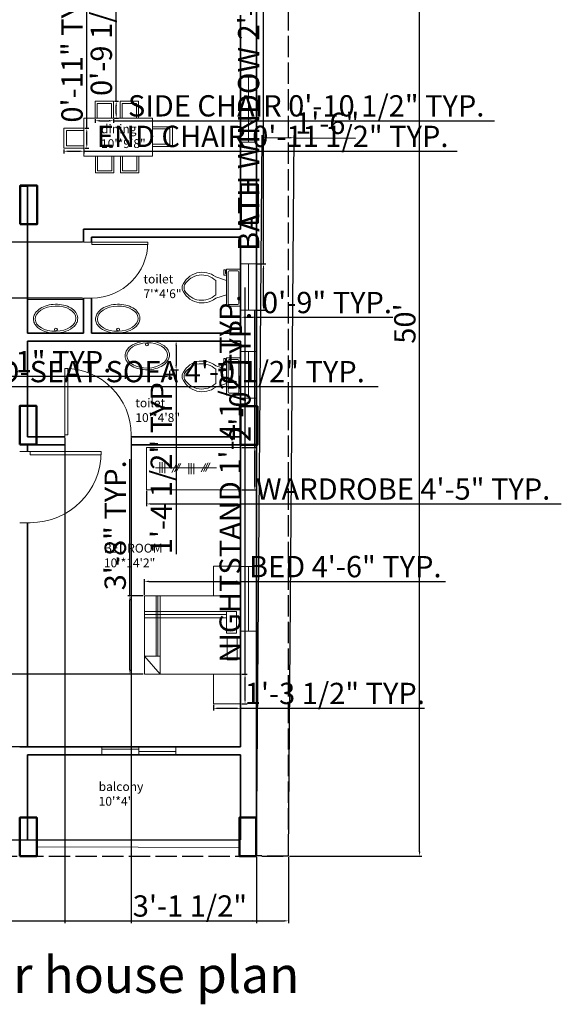
# Model space of a CAD drawing. Units: inches. Extents: x 2147 to 2722, y 2048 to 2905.
# Tile 2 of 3: x 2417 to 2722, y 2048 to 2602. Entities that reach past the tile are written whole.
import ezdxf

# ---------------------------------------------------------------- set-up
doc = ezdxf.new("R2010")
doc.units = ezdxf.units.IN
doc.linetypes.add('ACAD_ISO02W100', pattern=[15, 12, -3])
for name, color, linetype, lineweight in [('A-ANNO-DIMS', 2, 'Continuous', 18), ('A-ANNO-TITL', 7, 'Continuous', 35), ('A-AREA-IDEN', 7, 'Continuous', 18), ('A-COLS', 7, 'Continuous', 50), ('A-COLS-PATT', 252, 'Continuous', 13), ('A-DOOR', 3, 'Continuous', 18), ('A-FLOR-CASE', 8, 'Continuous', 18), ('A-FLOR-FIXT', 9, 'Continuous', 18), ('A-FLOR-HRAL', 3, 'Continuous', 18), ('A-FURN', 8, 'Continuous', 18), ('A-GLAZ', 4, 'Continuous', 18), ('A-WALL', 7, 'Continuous', 35), ('C-PROP', 6, 'ACAD_ISO02W100', 25)]:
    doc.layers.add(name, color=color, linetype=linetype, lineweight=lineweight)
doc.styles.get("Standard").update_dxf_attribs({"font": 'arial.ttf'})
doc.dimstyles.new('ISO-25', dxfattribs={"dimtxt": 12, "dimasz": 2.5, "dimexe": 1.25, "dimexo": 0.625, "dimtad": 1, "dimdec": 0, "dimlunit": 4, "dimtxsty": 'Standard', "dimcen": 2.5, "dimadec": 0, "dimazin": 0, "dimtfac": 1, "dimtdec": 0, "dimtmove": 0, "dimatfit": 3, "dimfxl": 1, "dimarcsym": 0})

# ---------------------------------------------------------------- blocks, each defined once
blk = doc.blocks.new('*D1')
at = {"layer": 'A-ANNO-DIMS', "color": 0, "lineweight": -2, "transparency": 16777216}
for p, q in [((2569.22, 2730.99), (2643.73, 2730.99)), ((2642.48, 2133.49), (2642.48, 2728.49)), ((2569.22, 2130.99), (2643.73, 2130.99))]:
    blk.add_line(p, q, dxfattribs=at)
at = {"layer": 'A-ANNO-DIMS', "color": 0, "lineweight": 100, "transparency": 16777216}
for points in [[(2642.06, 2728.49), (2642.9, 2728.49), (2642.48, 2730.99)], [(2642.06, 2133.49), (2642.9, 2133.49), (2642.48, 2130.99)]]:
    blk.add_solid(points, dxfattribs=at)
at = {"layer": 'Defpoints', "color": 0, "lineweight": 100, "transparency": 16777216}
for p in [(2568.6, 2730.99), (2642.48, 2730.99), (2568.6, 2130.99)]:
    blk.add_point(p, dxfattribs=at)
at = {"layer": 'A-ANNO-DIMS', "color": 0, "transparency": 16777216, "insert": (2635.73, 2430.99), "char_height": 12, "attachment_point": 5, "rotation": 90}
blk.add_mtext("50'", dxfattribs=at)
blk = doc.blocks.new('*U5')
for p, q in [((9.5, -6), (9.5, -2)), ((-10, -8.5), (-8, -8.5)), ((-10, -9.5), (-10, -8.5)), ((-7, -9.5), (-10, -9.5)), ((-8, -8.5), (-8, -8)), ((-7, -8), (-7, -9.5)), ((-4, -8), (-6, -14)), ((4, -8), (6, -14)), ((4, -14), (-4, -14))]:
    blk.add_line(p, q)
blk.add_lwpolyline([(10.5, -8), (10.5, 0), (-10.5, 0), (-10.5, -8)], close=True)
for points in [[(-9.5, -2), (-9.5, -6)], [(8.5, -1), (-8.5, -1)], [(-8.5, -7), (8.5, -7)]]:
    blk.add_lwpolyline(points)
for centre, radius, start, end in [((-8.62, -1.88), 0.884, 81.8699, 188.1301), ((8.62, -1.88), 0.884, 351.8699, 98.1301), ((-8.62, -6.12), 0.884, 171.8699, 278.1301), ((8.62, -6.12), 0.884, 261.8699, 8.1301), ((3.52, -21.58), 12.17, 141.4691, 247.9714), ((4.2, -21.82), 11.33, 136.3677, 238.9468), ((-3.52, -21.58), 12.17, 292.0284, 38.5307), ((-4.2, -21.82), 11.33, 301.053, 43.6321), ((0, -27.88), 4, 245.7318, 294.2682), ((0, -29), 4, 254.8605, 285.1395)]:
    blk.add_arc(centre, radius, start, end)
blk = doc.blocks.new('*U3')
for p, q in [((0, 0), (0, -6)), ((40, 0), (40, -6))]:
    blk.add_line(p, q)
blk.add_lwpolyline([(0, 0), (0, 40), (1.75, 40), (1.75, 0)], close=True)
blk.add_arc((0, 0), 40, 0, 90)
blk = doc.blocks.new('*D8')
at = {"layer": 'A-ANNO-DIMS', "color": 0, "lineweight": -2, "transparency": 16777216}
for p, q in [((2550.6, 2131.76), (2553.81, 2537.03)), ((2556.3, 2535.76), (2569.3, 2535.66)), ((2568.6, 2131.61), (2571.81, 2536.89)), ((2571.8, 2535.64), (2606.32, 2535.36))]:
    blk.add_line(p, q, dxfattribs=at)
at = {"layer": 'A-ANNO-DIMS', "color": 0, "lineweight": 100, "transparency": 16777216}
for points in [[(2556.3, 2536.17), (2556.3, 2535.34), (2553.8, 2535.78)], [(2569.3, 2536.07), (2569.3, 2535.24), (2571.8, 2535.64)]]:
    blk.add_solid(points, dxfattribs=at)
at = {"layer": 'Defpoints', "color": 0, "lineweight": 100, "transparency": 16777216}
for p in [(2571.8, 2535.64), (2550.6, 2131.13), (2568.6, 2130.99)]:
    blk.add_point(p, dxfattribs=at)
at = {"layer": 'A-ANNO-DIMS', "color": 0, "transparency": 16777216, "insert": (2590.36, 2542.24), "char_height": 12, "attachment_point": 5, "rotation": 359.5465}
blk.add_mtext('1\'-6"', dxfattribs=at)
blk = doc.blocks.new('BED-TWIN-PILLOW')
for p, q in [((6.6, 10.17), (6.6, 44.18)), ((7.66, 10.17), (7.66, 44.18)), ((8.88, 10.17), (8.88, 44.18)), ((46.28, 35.34), (0, 35.34)), ((46.28, 33.66), (0, 33.66)), ((46.28, 31.83), (0, 31.83)), ((8.88, 0), (0, 10.17))]:
    blk.add_line(p, q)
for points in [[(54.22, 44.18), (0, 44.18), (0, 0), (54.22, 0)], [(51.93, 35.34), (46.28, 35.34), (46.28, 23.14), (51.93, 23.14)], [(52.24, 20.39), (46.59, 20.39), (46.59, 8.19), (52.24, 8.19)], [(0, 0), (8.88, 0), (8.88, 10.17), (0, 10.17)]]:
    blk.add_lwpolyline(points, close=True)
blk = doc.blocks.new('NIGHTSTAND')
blk.add_lwpolyline([(15.28, 0), (0, 0), (0, 16.69), (15.28, 16.69)], close=True)
blk = doc.blocks.new('WARDROBE')
for p, q in [((5.01, 12.45), (39.39, 12.45)), ((7.59, 9.5), (7.59, 15.59)), ((8.92, 9.5), (8.92, 15.59)), ((10.35, 9.4), (10.35, 15.5)), ((14.36, 9.78), (16.93, 14.55)), ((15.74, 10.07), (18.32, 14.83)), ((16.79, 10.07), (19.36, 14.83)), ((23.89, 8.83), (23.89, 14.93)), ((25.23, 8.83), (25.23, 14.93)), ((26.66, 8.73), (26.66, 14.83)), ((30.8, 10.05), (33.37, 14.82)), ((32.18, 10.34), (34.76, 15.1)), ((33.23, 10.34), (35.81, 15.1))]:
    blk.add_line(p, q)
blk.add_lwpolyline([(53.03, 23.8), (0, 23.8), (0, 0), (53.03, 0)], close=True)
blk = doc.blocks.new('DINING-CHAIR')
for p, q in [((0, 0), (0, 9.48)), ((0, 9.48), (10.32, 9.48)), ((10.32, 9.48), (10.32, 0))]:
    blk.add_line(p, q)
blk.add_lwpolyline([(1.15, 0), (9.29, 0), (9.29, 8.23), (1.15, 8.23)], close=True)
blk = doc.blocks.new('DINING-END-CHAIR')
for p, q in [((11.3, 11.23), (0, 11.23)), ((0, 11.23), (0, 0)), ((0, 0), (11.3, 0))]:
    blk.add_line(p, q)
blk.add_lwpolyline([(11.3, 10.08), (1.54, 10.08), (1.54, 1.35), (11.3, 1.35)], close=True)
blk = doc.blocks.new('LAVATORY-OVAL')
blk.add_circle((12.66, 1.92), 0.807)
blk.add_ellipse((12.48, 8.1), major_axis=(11.49, 0.3), ratio=0.618261)
blk.add_open_spline([(24.96, 8.42), (24.94, 8.99), (24.84, 9.56), (24.46, 10.65), (24.18, 11.17), (23.14, 12.64), (22.17, 13.49), (19.82, 14.86), (18.46, 15.39), (15.51, 16.07), (13.93, 16.23), (10.78, 16.16), (9.21, 15.94), (6.29, 15.13), (4.94, 14.54), (2.64, 13.07), (1.69, 12.19), (0.58, 10.5), (0.27, 9.77), (-0.04, 8.25), (-0.04, 7.47), (0.3, 5.96), (0.63, 5.24), (1.56, 3.91), (2.16, 3.3), (4.19, 1.74), (5.92, 0.97), (9.73, 0.04), (11.82, -0.1), (15.89, 0.25), (17.87, 0.74), (21.27, 2.3), (22.7, 3.36), (24.16, 5.29), (24.54, 6.02), (24.9, 7.32), (24.97, 7.87), (24.96, 8.42)], degree=3, knots=[0, 0, 0, 0, 0.196222, 0.196222, 0.392443, 0.392443, 0.782806, 0.782806, 1.173169, 1.173169, 1.563532, 1.563532, 1.953895, 1.953895, 2.344257, 2.344257, 2.73462, 2.73462, 2.999289, 2.999289, 3.263958, 3.263958, 3.528626, 3.528626, 3.793295, 3.793295, 4.301198, 4.301198, 4.809101, 4.809101, 5.317004, 5.317004, 5.824907, 5.824907, 6.093414, 6.093414, 6.283185, 6.283185, 6.283185, 6.283185])
blk = doc.blocks.new('WINDOW-EXTERIOR')
blk.add_line((4.5, 36.51), (4.5, 0))
blk.add_lwpolyline([(0, 36.51), (9, 36.51), (9, 0), (0, 0)], close=True)
blk = doc.blocks.new('WINDOW-BATH')
blk.add_line((4.5, 26.12), (4.5, 0))
blk.add_lwpolyline([(0, 26.12), (9, 26.12), (9, 0), (0, 0)], close=True)
blk = doc.blocks.new('COLUMN-RECT')
blk.add_lwpolyline([(0, 0), (9.48, 0), (9.48, 21.75), (0, 21.75)], close=True)
blk = doc.blocks.new('*D22')
at = {"layer": 'A-ANNO-DIMS', "color": 0, "lineweight": -2, "transparency": 16777216}
for p, q in [((2544.1, 2233.45), (2544.1, 2451.35)), ((2542.22, 2233.45), (2545.35, 2233.45)), ((2544.1, 2219.26), (2544.1, 2230.95)), ((2542.22, 2216.76), (2545.35, 2216.76))]:
    blk.add_line(p, q, dxfattribs=at)
at = {"layer": 'A-ANNO-DIMS', "color": 0, "lineweight": 100, "transparency": 16777216}
for points in [[(2543.68, 2230.95), (2544.51, 2230.95), (2544.1, 2233.45)], [(2543.68, 2219.26), (2544.51, 2219.26), (2544.1, 2216.76)]]:
    blk.add_solid(points, dxfattribs=at)
at = {"layer": 'Defpoints', "color": 0, "lineweight": 100, "transparency": 16777216}
for p in [(2541.59, 2233.45), (2544.1, 2233.45), (2541.59, 2216.76)]:
    blk.add_point(p, dxfattribs=at)
at = {"layer": 'A-ANNO-DIMS', "color": 0, "transparency": 16777216, "insert": (2537.27, 2343.65), "char_height": 12, "attachment_point": 5, "rotation": 90}
blk.add_mtext('NIGHTSTAND 1\'-4 1/2" TYP.', dxfattribs=at)
blk = doc.blocks.new('*D23')
at = {"layer": 'A-ANNO-DIMS', "color": 0, "lineweight": -2, "transparency": 16777216}
for p, q in [((2526.32, 2216.14), (2526.32, 2213.01)), ((2528.82, 2214.26), (2539.09, 2214.26)), ((2541.59, 2216.14), (2541.59, 2213.01)), ((2541.59, 2214.26), (2645.32, 2214.26))]:
    blk.add_line(p, q, dxfattribs=at)
at = {"layer": 'A-ANNO-DIMS', "color": 0, "lineweight": 100, "transparency": 16777216}
for points in [[(2528.82, 2214.67), (2528.82, 2213.84), (2526.32, 2214.26)], [(2539.09, 2214.67), (2539.09, 2213.84), (2541.59, 2214.26)]]:
    blk.add_solid(points, dxfattribs=at)
at = {"layer": 'Defpoints', "color": 0, "lineweight": 100, "transparency": 16777216}
for p in [(2526.32, 2216.76), (2541.59, 2216.76), (2541.59, 2214.26)]:
    blk.add_point(p, dxfattribs=at)
at = {"layer": 'A-ANNO-DIMS', "color": 0, "transparency": 16777216, "insert": (2594.71, 2221.09), "char_height": 12, "attachment_point": 5}
blk.add_mtext('1\'-3 1/2" TYP.', dxfattribs=at)
blk = doc.blocks.new('*D24')
at = {"layer": 'A-ANNO-DIMS', "color": 0, "lineweight": -2, "transparency": 16777216}
for p, q in [((2459.63, 2546.14), (2459.63, 2543.97)), ((2469.94, 2546.14), (2469.94, 2543.97)), ((2462.13, 2545.22), (2467.44, 2545.22)), ((2469.94, 2545.22), (2684.67, 2545.22))]:
    blk.add_line(p, q, dxfattribs=at)
at = {"layer": 'A-ANNO-DIMS', "color": 0, "lineweight": 100, "transparency": 16777216}
for points in [[(2462.13, 2545.63), (2462.13, 2544.8), (2459.63, 2545.22)], [(2467.44, 2545.63), (2467.44, 2544.8), (2469.94, 2545.22)]]:
    blk.add_solid(points, dxfattribs=at)
at = {"layer": 'Defpoints', "color": 0, "lineweight": 100, "transparency": 16777216}
for p in [(2459.63, 2546.76), (2469.94, 2546.76), (2469.94, 2545.22)]:
    blk.add_point(p, dxfattribs=at)
at = {"layer": 'A-ANNO-DIMS', "color": 0, "transparency": 16777216, "insert": (2578.56, 2552.05), "char_height": 12, "attachment_point": 5}
blk.add_mtext('SIDE CHAIR 0\'-10 1/2" TYP.', dxfattribs=at)
blk = doc.blocks.new('*D25')
at = {"layer": 'A-ANNO-DIMS', "color": 0, "lineweight": -2, "transparency": 16777216}
for p, q in [((2471.49, 2556.24), (2471.49, 2661.1)), ((2470.57, 2556.24), (2472.74, 2556.24)), ((2471.49, 2549.26), (2471.49, 2553.74)), ((2470.57, 2546.76), (2472.74, 2546.76))]:
    blk.add_line(p, q, dxfattribs=at)
at = {"layer": 'A-ANNO-DIMS', "color": 0, "lineweight": 100, "transparency": 16777216}
for points in [[(2471.08, 2553.74), (2471.91, 2553.74), (2471.49, 2556.24)], [(2471.08, 2549.26), (2471.91, 2549.26), (2471.49, 2546.76)]]:
    blk.add_solid(points, dxfattribs=at)
at = {"layer": 'Defpoints', "color": 0, "lineweight": 100, "transparency": 16777216}
for p in [(2469.94, 2556.24), (2471.49, 2556.24), (2469.94, 2546.76)]:
    blk.add_point(p, dxfattribs=at)
at = {"layer": 'A-ANNO-DIMS', "color": 0, "transparency": 16777216, "insert": (2464.66, 2609.92), "char_height": 12, "attachment_point": 5, "rotation": 90}
blk.add_mtext('0\'-9 1/2" TYP.', dxfattribs=at)
blk = doc.blocks.new('*D28')
at = {"layer": 'A-ANNO-DIMS', "color": 0, "lineweight": -2, "transparency": 16777216}
for p, q in [((2487.37, 2278.26), (2487.37, 2287.02)), ((2489.87, 2285.77), (2539.09, 2285.77)), ((2541.59, 2278.26), (2541.59, 2287.02)), ((2541.59, 2285.77), (2657.08, 2285.77))]:
    blk.add_line(p, q, dxfattribs=at)
at = {"layer": 'A-ANNO-DIMS', "color": 0, "lineweight": 100, "transparency": 16777216}
for points in [[(2489.87, 2286.18), (2489.87, 2285.35), (2487.37, 2285.77)], [(2539.09, 2286.18), (2539.09, 2285.35), (2541.59, 2285.77)]]:
    blk.add_solid(points, dxfattribs=at)
at = {"layer": 'Defpoints', "color": 0, "lineweight": 100, "transparency": 16777216}
for p in [(2541.59, 2285.77), (2487.37, 2277.63), (2541.59, 2277.63)]:
    blk.add_point(p, dxfattribs=at)
at = {"layer": 'A-ANNO-DIMS', "color": 0, "transparency": 16777216, "insert": (2600.59, 2292.52), "char_height": 12, "attachment_point": 5}
blk.add_mtext('BED 4\'-6" TYP.', dxfattribs=at)
blk = doc.blocks.new('*D29')
at = {"layer": 'A-ANNO-DIMS', "color": 0, "lineweight": -2, "transparency": 16777216}
for p, q in [((2479.24, 2277.63), (2479.24, 2354.52)), ((2486.75, 2277.63), (2477.99, 2277.63)), ((2479.24, 2235.95), (2479.24, 2275.13)), ((2486.75, 2233.45), (2477.99, 2233.45))]:
    blk.add_line(p, q, dxfattribs=at)
at = {"layer": 'A-ANNO-DIMS', "color": 0, "lineweight": 100, "transparency": 16777216}
for points in [[(2478.82, 2275.13), (2479.66, 2275.13), (2479.24, 2277.63)], [(2478.82, 2235.95), (2479.66, 2235.95), (2479.24, 2233.45)]]:
    blk.add_solid(points, dxfattribs=at)
at = {"layer": 'Defpoints', "color": 0, "lineweight": 100, "transparency": 16777216}
for p in [(2479.24, 2277.63), (2487.37, 2277.63), (2487.37, 2233.45)]:
    blk.add_point(p, dxfattribs=at)
at = {"layer": 'A-ANNO-DIMS', "color": 0, "transparency": 16777216, "insert": (2472.48, 2317.33), "char_height": 12, "attachment_point": 5, "rotation": 90}
blk.add_mtext('3\'-8" TYP.', dxfattribs=at)
blk = doc.blocks.new('*D30')
at = {"layer": 'A-ANNO-DIMS', "color": 0, "lineweight": -2, "transparency": 16777216}
for p, q in [((2476.51, 2404.28), (2476.51, 2399.9)), ((2501.53, 2404.28), (2501.53, 2399.9)), ((2476.51, 2401.15), (2295.38, 2401.15)), ((2499.03, 2401.15), (2479.01, 2401.15))]:
    blk.add_line(p, q, dxfattribs=at)
at = {"layer": 'A-ANNO-DIMS', "color": 0, "lineweight": 100, "transparency": 16777216}
for points in [[(2479.01, 2401.57), (2479.01, 2400.73), (2476.51, 2401.15)], [(2499.03, 2401.57), (2499.03, 2400.73), (2501.53, 2401.15)]]:
    blk.add_solid(points, dxfattribs=at)
at = {"layer": 'Defpoints', "color": 0, "lineweight": 100, "transparency": 16777216}
for p in [(2476.51, 2404.9), (2501.53, 2404.9), (2476.51, 2401.15)]:
    blk.add_point(p, dxfattribs=at)
at = {"layer": 'A-ANNO-DIMS', "color": 0, "transparency": 16777216, "insert": (2384.7, 2407.98), "char_height": 12, "attachment_point": 5}
blk.add_mtext('OVAL BASIN 2\'-1" TYP.', dxfattribs=at)
blk = doc.blocks.new('*D31')
at = {"layer": 'A-ANNO-DIMS', "color": 0, "lineweight": -2, "transparency": 16777216}
for p, q in [((2502.15, 2421.24), (2506.53, 2421.24)), ((2505.28, 2418.74), (2505.28, 2407.4)), ((2502.15, 2404.9), (2506.53, 2404.9)), ((2505.28, 2404.9), (2505.28, 2301.17))]:
    blk.add_line(p, q, dxfattribs=at)
at = {"layer": 'A-ANNO-DIMS', "color": 0, "lineweight": 100, "transparency": 16777216}
for points in [[(2504.87, 2418.74), (2505.7, 2418.74), (2505.28, 2421.24)], [(2504.87, 2407.4), (2505.7, 2407.4), (2505.28, 2404.9)]]:
    blk.add_solid(points, dxfattribs=at)
at = {"layer": 'Defpoints', "color": 0, "lineweight": 100, "transparency": 16777216}
for p in [(2501.53, 2421.24), (2501.53, 2404.9), (2505.28, 2404.9)]:
    blk.add_point(p, dxfattribs=at)
at = {"layer": 'A-ANNO-DIMS', "color": 0, "transparency": 16777216, "insert": (2498.45, 2351.79), "char_height": 12, "attachment_point": 5, "rotation": 90}
blk.add_mtext('1\'-4 1/2" TYP.', dxfattribs=at)
blk = doc.blocks.new('*D34')
at = {"layer": 'A-ANNO-DIMS', "color": 0, "lineweight": -2, "transparency": 16777216}
for p, q in [((2488.57, 2336.73), (2488.57, 2328.15)), ((2541.59, 2336.73), (2541.59, 2328.15)), ((2491.07, 2329.4), (2539.09, 2329.4)), ((2541.59, 2329.4), (2722.36, 2329.4))]:
    blk.add_line(p, q, dxfattribs=at)
at = {"layer": 'A-ANNO-DIMS', "color": 0, "lineweight": 100, "transparency": 16777216}
for points in [[(2491.07, 2329.81), (2491.07, 2328.98), (2488.57, 2329.4)], [(2539.09, 2329.81), (2539.09, 2328.98), (2541.59, 2329.4)]]:
    blk.add_solid(points, dxfattribs=at)
at = {"layer": 'Defpoints', "color": 0, "lineweight": 100, "transparency": 16777216}
for p in [(2488.57, 2337.35), (2541.59, 2337.35), (2541.59, 2329.4)]:
    blk.add_point(p, dxfattribs=at)
at = {"layer": 'A-ANNO-DIMS', "color": 0, "transparency": 16777216, "insert": (2633.23, 2336.23), "char_height": 12, "attachment_point": 5}
blk.add_mtext('WARDROBE 4\'-5" TYP.', dxfattribs=at)
blk = doc.blocks.new('*D35')
at = {"layer": 'A-ANNO-DIMS', "color": 0, "lineweight": -2, "transparency": 16777216}
for p, q in [((2549.55, 2361.15), (2549.55, 2438.25)), ((2542.22, 2361.15), (2550.8, 2361.15)), ((2549.55, 2339.85), (2549.55, 2358.65)), ((2542.22, 2337.35), (2550.8, 2337.35))]:
    blk.add_line(p, q, dxfattribs=at)
at = {"layer": 'A-ANNO-DIMS', "color": 0, "lineweight": 100, "transparency": 16777216}
for points in [[(2549.13, 2358.65), (2549.96, 2358.65), (2549.55, 2361.15)], [(2549.13, 2339.85), (2549.96, 2339.85), (2549.55, 2337.35)]]:
    blk.add_solid(points, dxfattribs=at)
at = {"layer": 'Defpoints', "color": 0, "lineweight": 100, "transparency": 16777216}
for p in [(2541.59, 2361.15), (2549.55, 2361.15), (2541.59, 2337.35)]:
    blk.add_point(p, dxfattribs=at)
at = {"layer": 'A-ANNO-DIMS', "color": 0, "transparency": 16777216, "insert": (2542.8, 2400.95), "char_height": 12, "attachment_point": 5, "rotation": 90}
blk.add_mtext('2\'-0" TYP.', dxfattribs=at)
blk = doc.blocks.new('*D36')
at = {"layer": 'A-ANNO-DIMS', "color": 0, "lineweight": -2, "transparency": 16777216}
for p, q in [((2441.9, 2529.1), (2441.9, 2526.78)), ((2453.21, 2529.1), (2453.21, 2526.78)), ((2444.4, 2528.03), (2450.71, 2528.03)), ((2453.21, 2528.03), (2663.62, 2528.03))]:
    blk.add_line(p, q, dxfattribs=at)
at = {"layer": 'A-ANNO-DIMS', "color": 0, "lineweight": 100, "transparency": 16777216}
for points in [[(2444.4, 2528.45), (2444.4, 2527.62), (2441.9, 2528.03)], [(2450.71, 2528.45), (2450.71, 2527.62), (2453.21, 2528.03)]]:
    blk.add_solid(points, dxfattribs=at)
at = {"layer": 'Defpoints', "color": 0, "lineweight": 100, "transparency": 16777216}
for p in [(2441.9, 2529.73), (2453.21, 2529.73), (2453.21, 2528.03)]:
    blk.add_point(p, dxfattribs=at)
at = {"layer": 'A-ANNO-DIMS', "color": 0, "transparency": 16777216, "insert": (2559.66, 2534.86), "char_height": 12, "attachment_point": 5}
blk.add_mtext('END CHAIR 0\'-11 1/2" TYP.', dxfattribs=at)
blk = doc.blocks.new('*D37')
at = {"layer": 'A-ANNO-DIMS', "color": 0, "lineweight": -2, "transparency": 16777216}
for p, q in [((2454.9, 2540.96), (2454.9, 2627.18)), ((2453.83, 2540.96), (2456.15, 2540.96)), ((2454.9, 2532.23), (2454.9, 2538.46)), ((2453.83, 2529.73), (2456.15, 2529.73))]:
    blk.add_line(p, q, dxfattribs=at)
at = {"layer": 'A-ANNO-DIMS', "color": 0, "lineweight": 100, "transparency": 16777216}
for points in [[(2454.48, 2538.46), (2455.32, 2538.46), (2454.9, 2540.96)], [(2454.48, 2532.23), (2455.32, 2532.23), (2454.9, 2529.73)]]:
    blk.add_solid(points, dxfattribs=at)
at = {"layer": 'Defpoints', "color": 0, "lineweight": 100, "transparency": 16777216}
for p in [(2453.21, 2540.96), (2454.9, 2540.96), (2453.21, 2529.73)]:
    blk.add_point(p, dxfattribs=at)
at = {"layer": 'A-ANNO-DIMS', "color": 0, "transparency": 16777216, "insert": (2448.15, 2585.32), "char_height": 12, "attachment_point": 5, "rotation": 90}
blk.add_mtext('0\'-11" TYP.', dxfattribs=at)
blk = doc.blocks.new('*D38')
at = {"layer": 'A-ANNO-DIMS', "color": 0, "lineweight": -2, "transparency": 16777216}
for p, q in [((2321.88, 2402.21), (2321.88, 2394.28)), ((2370.6, 2402.21), (2370.6, 2394.28)), ((2324.38, 2395.53), (2368.1, 2395.53)), ((2370.6, 2395.53), (2619.19, 2395.53))]:
    blk.add_line(p, q, dxfattribs=at)
at = {"layer": 'A-ANNO-DIMS', "color": 0, "lineweight": 100, "transparency": 16777216}
for points in [[(2324.38, 2395.95), (2324.38, 2395.11), (2321.88, 2395.53)], [(2368.1, 2395.95), (2368.1, 2395.11), (2370.6, 2395.53)]]:
    blk.add_solid(points, dxfattribs=at)
at = {"layer": 'Defpoints', "color": 0, "lineweight": 100, "transparency": 16777216}
for p in [(2321.88, 2402.84), (2370.6, 2402.84), (2370.6, 2395.53)]:
    blk.add_point(p, dxfattribs=at)
at = {"layer": 'A-ANNO-DIMS', "color": 0, "transparency": 16777216, "insert": (2496.15, 2402.36), "char_height": 12, "attachment_point": 5}
blk.add_mtext('TWO-SEAT SOFA 4\'-0 1/2" TYP.', dxfattribs=at)
blk = doc.blocks.new('*D42')
at = {"layer": 'A-ANNO-DIMS', "color": 0, "lineweight": -2, "transparency": 16777216}
for p, q in [((2554.51, 2464.55), (2554.51, 2668.49)), ((2551.22, 2464.55), (2555.76, 2464.55)), ((2554.51, 2440.93), (2554.51, 2462.05)), ((2551.22, 2438.43), (2555.76, 2438.43))]:
    blk.add_line(p, q, dxfattribs=at)
at = {"layer": 'A-ANNO-DIMS', "color": 0, "lineweight": 100, "transparency": 16777216}
for points in [[(2554.1, 2462.05), (2554.93, 2462.05), (2554.51, 2464.55)], [(2554.1, 2440.93), (2554.93, 2440.93), (2554.51, 2438.43)]]:
    blk.add_solid(points, dxfattribs=at)
at = {"layer": 'Defpoints', "color": 0, "lineweight": 100, "transparency": 16777216}
for p in [(2550.6, 2464.55), (2554.51, 2464.55), (2550.6, 2438.43)]:
    blk.add_point(p, dxfattribs=at)
at = {"layer": 'A-ANNO-DIMS', "color": 0, "transparency": 16777216, "insert": (2547.68, 2567.77), "char_height": 12, "attachment_point": 5, "rotation": 90}
blk.add_mtext('BATH WINDOW 2\'-2" TYP.', dxfattribs=at)
blk = doc.blocks.new('*D43')
at = {"layer": 'A-ANNO-DIMS', "color": 0, "lineweight": -2, "transparency": 16777216}
for p, q in [((2541.59, 2437.81), (2541.59, 2433.27)), ((2550.6, 2437.81), (2550.6, 2433.27)), ((2544.09, 2434.52), (2548.1, 2434.52)), ((2550.6, 2434.52), (2627.49, 2434.52))]:
    blk.add_line(p, q, dxfattribs=at)
at = {"layer": 'A-ANNO-DIMS', "color": 0, "lineweight": 100, "transparency": 16777216}
for points in [[(2544.09, 2434.93), (2544.09, 2434.1), (2541.59, 2434.52)], [(2548.1, 2434.93), (2548.1, 2434.1), (2550.6, 2434.52)]]:
    blk.add_solid(points, dxfattribs=at)
at = {"layer": 'Defpoints', "color": 0, "lineweight": 100, "transparency": 16777216}
for p in [(2541.59, 2438.43), (2550.6, 2438.43), (2550.6, 2434.52)]:
    blk.add_point(p, dxfattribs=at)
at = {"layer": 'A-ANNO-DIMS', "color": 0, "transparency": 16777216, "insert": (2590.3, 2441.27), "char_height": 12, "attachment_point": 5}
blk.add_mtext('0\'-9" TYP.', dxfattribs=at)
blk = doc.blocks.new('*D46')
at = {"layer": 'A-ANNO-DIMS', "color": 0, "lineweight": -2, "transparency": 16777216}
for p, q in [((2208.6, 2130.36), (2208.6, 2093.29)), ((2568.6, 2130.36), (2568.6, 2093.29)), ((2211.1, 2094.54), (2566.1, 2094.54))]:
    blk.add_line(p, q, dxfattribs=at)
at = {"layer": 'A-ANNO-DIMS', "color": 0, "lineweight": 100, "transparency": 16777216}
for points in [[(2211.1, 2094.96), (2211.1, 2094.12), (2208.6, 2094.54)], [(2566.1, 2094.96), (2566.1, 2094.12), (2568.6, 2094.54)]]:
    blk.add_solid(points, dxfattribs=at)
at = {"layer": 'Defpoints', "color": 0, "lineweight": 100, "transparency": 16777216}
for p in [(2208.6, 2130.99), (2568.6, 2130.99), (2568.6, 2094.54)]:
    blk.add_point(p, dxfattribs=at)
at = {"layer": 'A-ANNO-DIMS', "color": 0, "transparency": 16777216, "insert": (2388.6, 2101.3), "char_height": 12, "attachment_point": 5}
blk.add_mtext('30\'-0"', dxfattribs=at)
blk = doc.blocks.new('*D47')
at = {"layer": 'A-ANNO-DIMS', "color": 0, "lineweight": -2, "transparency": 16777216}
for p, q in [((2220.6, 2130.36), (2220.6, 2093.29)), ((2550.6, 2130.51), (2550.6, 2093.29)), ((2223.1, 2094.54), (2548.1, 2094.54))]:
    blk.add_line(p, q, dxfattribs=at)
at = {"layer": 'A-ANNO-DIMS', "color": 0, "lineweight": 100, "transparency": 16777216}
for points in [[(2223.1, 2094.96), (2223.1, 2094.12), (2220.6, 2094.54)], [(2548.1, 2094.96), (2548.1, 2094.12), (2550.6, 2094.54)]]:
    blk.add_solid(points, dxfattribs=at)
at = {"layer": 'Defpoints', "color": 0, "lineweight": 100, "transparency": 16777216}
for p in [(2220.6, 2130.99), (2550.6, 2131.13), (2550.6, 2094.54)]:
    blk.add_point(p, dxfattribs=at)
at = {"layer": 'A-ANNO-DIMS', "color": 0, "transparency": 16777216, "insert": (2385.6, 2101.29), "char_height": 12, "attachment_point": 5}
blk.add_mtext('27\'-6"', dxfattribs=at)
blk = doc.blocks.new('*D50')
at = {"layer": 'A-ANNO-DIMS', "color": 0, "lineweight": -2, "transparency": 16777216}
for p, q in [((2486.75, 2233.45), (2170.9, 2233.45)), ((2172.15, 2230.95), (2172.15, 2195.13)), ((2483.59, 2192.63), (2170.9, 2192.63))]:
    blk.add_line(p, q, dxfattribs=at)
at = {"layer": 'A-ANNO-DIMS', "color": 0, "lineweight": 100, "transparency": 16777216}
for points in [[(2171.73, 2230.95), (2172.56, 2230.95), (2172.15, 2233.45)], [(2171.73, 2195.13), (2172.56, 2195.13), (2172.15, 2192.63)]]:
    blk.add_solid(points, dxfattribs=at)
at = {"layer": 'Defpoints', "color": 0, "lineweight": 100, "transparency": 16777216}
for p in [(2487.37, 2233.45), (2172.15, 2192.63), (2484.21, 2192.63)]:
    blk.add_point(p, dxfattribs=at)
at = {"layer": 'A-ANNO-DIMS', "color": 0, "transparency": 16777216, "insert": (2165.39, 2213.04), "char_height": 12, "attachment_point": 5, "rotation": 90}
blk.add_mtext('3\'-5"', dxfattribs=at)
blk = doc.blocks.new('*D51')
at = {"layer": 'A-ANNO-DIMS', "color": 0, "lineweight": -2, "transparency": 16777216}
for p, q in [((2172.15, 2476.87), (2172.15, 2540.69)), ((2452.47, 2476.87), (2170.9, 2476.87)), ((2172.15, 2447.87), (2172.15, 2474.37)), ((2452.47, 2445.37), (2170.9, 2445.37))]:
    blk.add_line(p, q, dxfattribs=at)
at = {"layer": 'A-ANNO-DIMS', "color": 0, "lineweight": 100, "transparency": 16777216}
for points in [[(2171.73, 2474.37), (2172.56, 2474.37), (2172.15, 2476.87)], [(2171.73, 2447.87), (2172.56, 2447.87), (2172.15, 2445.37)]]:
    blk.add_solid(points, dxfattribs=at)
at = {"layer": 'Defpoints', "color": 0, "lineweight": 100, "transparency": 16777216}
for p in [(2172.15, 2476.87), (2453.09, 2476.87), (2453.09, 2445.37)]:
    blk.add_point(p, dxfattribs=at)
at = {"layer": 'A-ANNO-DIMS', "color": 0, "transparency": 16777216, "insert": (2165.32, 2510.03), "char_height": 12, "attachment_point": 5, "rotation": 90}
blk.add_mtext('2\'-7 1/2"', dxfattribs=at)
blk = doc.blocks.new('*D52')
at = {"layer": 'A-ANNO-DIMS', "color": 0, "lineweight": -2, "transparency": 16777216}
for p, q in [((2442.63, 2366.51), (2442.63, 2093.29)), ((2479.99, 2366.51), (2479.99, 2093.29)), ((2445.13, 2094.54), (2477.49, 2094.54)), ((2479.99, 2094.54), (2543.59, 2094.54))]:
    blk.add_line(p, q, dxfattribs=at)
at = {"layer": 'A-ANNO-DIMS', "color": 0, "lineweight": 100, "transparency": 16777216}
for points in [[(2445.13, 2094.96), (2445.13, 2094.12), (2442.63, 2094.54)], [(2477.49, 2094.96), (2477.49, 2094.12), (2479.99, 2094.54)]]:
    blk.add_solid(points, dxfattribs=at)
at = {"layer": 'Defpoints', "color": 0, "lineweight": 100, "transparency": 16777216}
for p in [(2442.63, 2367.13), (2479.99, 2367.13), (2479.99, 2094.54)]:
    blk.add_point(p, dxfattribs=at)
at = {"layer": 'A-ANNO-DIMS', "color": 0, "transparency": 16777216, "insert": (2513.04, 2101.37), "char_height": 12, "attachment_point": 5}
blk.add_mtext('3\'-1 1/2"', dxfattribs=at)

msp = doc.modelspace()

# ---------------------------------------------------------------- hatches: boundary and pattern name
at = {"layer": 'A-COLS-PATT'}
h = msp.add_hatch(dxfattribs=at)
h.set_pattern_fill('AR-SAND', color=256, scale=5)
h.paths.add_polyline_path([(2439.24, 2712.96), (2417.09, 2712.96), (2417.09, 2703.96), (2421.59, 2703.96), (2421.59, 2703.99), (2439.24, 2703.99)])
h.paths.add_polyline_path([(2550.6, 2712.99), (2528.45, 2712.99), (2528.45, 2703.99), (2541.27, 2703.99), (2550.6, 2703.99)])
h.paths.add_polyline_path([(2229.6, 2593.61), (2220.6, 2593.61), (2220.6, 2571.86), (2229.6, 2571.86), (2229.6, 2574.49), (2230.08, 2574.49), (2230.08, 2578.99), (2229.6, 2578.99)])
h.paths.add_polyline_path([(2229.6, 2152.74), (2220.6, 2152.74), (2220.6, 2130.99), (2229.6, 2130.99), (2230.08, 2130.99), (2230.08, 2139.99), (2229.6, 2139.99)])
h.paths.add_polyline_path([(2301.09, 2152.74), (2296.59, 2152.74), (2296.59, 2140.02), (2301.09, 2140.03)])
h.paths.add_polyline_path([(2306.03, 2152.74), (2301.09, 2152.74), (2301.09, 2140.03), (2306.03, 2140.03)])
h.paths.add_polyline_path([(2306.03, 2140.03), (2296.55, 2140.02), (2296.55, 2130.99), (2306.03, 2130.99)])
h.paths.add_polyline_path([(2426.67, 2152.74), (2421.59, 2152.74), (2421.59, 2140.08), (2426.67, 2140.08)])
h.paths.add_polyline_path([(2421.59, 2152.74), (2417.19, 2152.74), (2417.19, 2140.08), (2421.59, 2140.08)])
h.paths.add_polyline_path([(2426.67, 2140.08), (2421.59, 2140.08), (2417.19, 2140.08), (2417.19, 2130.99), (2426.67, 2130.99)])
h = msp.add_hatch(dxfattribs=at)
h.set_pattern_fill('AR-SAND', color=256, scale=5)
h.paths.add_polyline_path([(2550.6, 2384.38), (2541.59, 2384.38), (2541.59, 2362.63), (2550.6, 2362.63)])
h.paths.add_polyline_path([(2426.57, 2384.56), (2421.59, 2384.56), (2421.59, 2367.13), (2426.57, 2367.13)], flags=17)
h.paths.add_polyline_path([(2421.59, 2384.56), (2417.09, 2384.56), (2417.09, 2362.81), (2426.57, 2362.81), (2426.57, 2367.13), (2421.59, 2367.13)])
h.paths.add_polyline_path([(2550.39, 2152.74), (2541.59, 2152.74), (2541.59, 2140.13), (2540.91, 2140.13), (2540.91, 2130.99), (2550.39, 2130.99)])
h.paths.add_polyline_path([(2361.09, 2353.99), (2343.4, 2353.99), (2343.4, 2349.49), (2361.09, 2349.49)], flags=17)
h.paths.add_polyline_path([(2365.55, 2358.49), (2343.4, 2358.49), (2343.4, 2353.99), (2361.09, 2353.99), (2361.09, 2349.49), (2365.55, 2349.49)])
h.paths.add_polyline_path([(2550.6, 2509.38), (2541.81, 2509.38), (2541.81, 2487.62), (2550.6, 2487.62)])
h.paths.add_polyline_path([(2229.6, 2370.15), (2220.6, 2370.15), (2220.6, 2348.39), (2229.6, 2348.39)])
h.paths.add_polyline_path([(2426.88, 2508.65), (2417.4, 2508.65), (2417.4, 2508.45), (2421.59, 2508.45), (2421.59, 2486.9), (2426.88, 2486.9)])
h.paths.add_polyline_path([(2421.59, 2508.45), (2417.4, 2508.45), (2417.4, 2486.9), (2421.59, 2486.9)], flags=17)

# ---------------------------------------------------------------- linework, layer by layer
at = {"layer": 'A-COLS'}
for points in [[(2417.4, 2486.9), (2426.88, 2486.9), (2426.88, 2508.65), (2417.4, 2508.65)], [(2541.81, 2487.62), (2551.29, 2487.62), (2551.29, 2509.38), (2541.81, 2509.38)], [(2417.09, 2362.81), (2426.57, 2362.81), (2426.57, 2384.56), (2417.09, 2384.56)], [(2541.59, 2362.63), (2551.07, 2362.63), (2551.07, 2384.38), (2541.59, 2384.38)], [(2540.91, 2130.99), (2550.39, 2130.99), (2550.39, 2152.74), (2540.91, 2152.74)]]:
    msp.add_lwpolyline(points, close=True, dxfattribs=at)
at = {"layer": 'A-DOOR'}
for p, q in [((2463.4, 2191.24), (2484.21, 2191.24)), ((2484.21, 2192.63), (2484.21, 2188.13)), ((2484.21, 2189.89), (2505.02, 2189.89))]:
    msp.add_line(p, q, dxfattribs=at)
msp.add_lwpolyline([(2463.4, 2192.63), (2505.02, 2192.63), (2505.02, 2188.13), (2463.4, 2188.13)], close=True, dxfattribs=at)
at = {"layer": 'A-FLOR-CASE'}
for p, q in [((2453.09, 2444.47), (2421.59, 2444.47)), ((2541.59, 2361.15), (2541.59, 2331.65))]:
    msp.add_line(p, q, dxfattribs=at)
at = {"layer": 'A-FLOR-HRAL'}
msp.add_line((2426.67, 2136.27), (2540.91, 2135.85), dxfattribs=at)
at = {"layer": 'A-FURN'}
msp.add_lwpolyline([(2453.21, 2546.76), (2491.97, 2546.76), (2491.97, 2525.27), (2453.21, 2525.27)], close=True, dxfattribs=at)
at = {"layer": 'A-WALL'}
for p, q in [((2550.6, 2131.13), (2550.6, 2712.99)), ((2541.59, 2604.63), (2541.59, 2580.48)), ((2541.59, 2484.13), (2541.59, 2600.13)), ((2541.59, 2484.13), (2541.59, 2600.13)), ((2417.09, 2508.45), (2421.59, 2508.45)), ((2421.59, 2508.45), (2421.59, 2484.13)), ((2421.59, 2484.13), (2421.59, 2503.37)), ((2421.59, 2484.13), (2421.59, 2467.39)), ((2421.59, 2425.63), (2421.59, 2479.63)), ((2541.59, 2484.13), (2453.09, 2484.13)), ((2453.09, 2479.63), (2453.09, 2484.13)), ((2453.09, 2479.63), (2453.09, 2476.87)), ((2541.59, 2479.63), (2457.59, 2479.63)), ((2457.59, 2479.63), (2457.59, 2476.87)), ((2541.59, 2425.63), (2541.59, 2479.63)), ((2453.09, 2445.37), (2453.09, 2425.63)), ((2457.59, 2445.37), (2457.59, 2425.63)), ((2453.09, 2425.63), (2421.59, 2425.63)), ((2541.59, 2425.63), (2457.59, 2425.63)), ((2541.59, 2421.13), (2421.59, 2421.13)), ((2421.59, 2421.13), (2421.59, 2367.13)), ((2541.59, 2367.13), (2541.59, 2421.13)), ((2442.63, 2367.13), (2421.59, 2367.13)), ((2421.59, 2362.63), (2421.59, 2358.83)), ((2442.63, 2362.63), (2421.59, 2362.63)), ((2541.59, 2367.13), (2479.99, 2367.13)), ((2541.59, 2362.63), (2479.99, 2362.63)), ((2541.59, 2192.63), (2541.59, 2362.63)), ((2421.59, 2318.83), (2421.59, 2192.63)), ((2541.59, 2192.63), (2417.09, 2192.63)), ((2541.59, 2188.13), (2421.59, 2188.13)), ((2421.59, 2188.13), (2421.59, 2140.13)), ((2541.59, 2140.13), (2541.59, 2188.13)), ((2229.6, 2139.99), (2541.59, 2140.13))]:
    msp.add_line(p, q, dxfattribs=at)
at = {"layer": 'C-PROP'}
msp.add_line((2568.6, 2130.99), (2550.6, 2131.13), dxfattribs=at)
msp.add_lwpolyline([(2208.6, 2130.99), (2568.6, 2130.99), (2568.6, 2730.99), (2208.6, 2730.99)], close=True, dxfattribs=at)

# ---------------------------------------------------------------- block references
at = {"layer": 'A-COLS'}
msp.add_blockref('COLUMN-RECT', (2417.19, 2130.99), dxfattribs=at)
at = {"layer": 'A-DOOR', "xscale": 0.7874895201585962, "yscale": 0.7874895201585962, "zscale": 0.7874895201585962, "rotation": 270}
msp.add_blockref('*U3', (2457.82, 2476.87), dxfattribs=at)
at = {"layer": 'A-DOOR', "xscale": 0.9339802048399524, "yscale": 0.9339802048399524, "zscale": 0.9339802048399524}
msp.add_blockref('*U3', (2442.63, 2368.24), dxfattribs=at)
at = {"layer": 'A-DOOR', "rotation": 270}
msp.add_blockref('*U3', (2423.09, 2358.83), dxfattribs=at)
at = {"layer": 'A-FLOR-CASE'}
msp.add_blockref('WARDROBE', (2488.57, 2337.35), dxfattribs=at)
at = {"layer": 'A-FLOR-FIXT'}
for name, p, rotation in [('*U5', (2541.59, 2451.21), 270), ('LAVATORY-OVAL', (2501.48, 2421.13), 180), ('*U5', (2541.59, 2401.23), 270)]:
    msp.add_blockref(name, p, dxfattribs=dict(at, rotation=rotation))
for p in [(2424.86, 2425.63), (2459.88, 2425.63)]:
    msp.add_blockref('LAVATORY-OVAL', p, dxfattribs=at)
at = {"layer": 'A-FURN'}
for name, p in [('DINING-CHAIR', (2459.63, 2546.76)), ('DINING-CHAIR', (2473.69, 2546.76)), ('DINING-END-CHAIR', (2441.9, 2529.73)), ('NIGHTSTAND', (2526.32, 2277.63)), ('BED-TWIN-PILLOW', (2487.37, 2233.45)), ('NIGHTSTAND', (2526.32, 2216.76))]:
    msp.add_blockref(name, p, dxfattribs=at)
at = {"layer": 'A-FURN', "extrusion": (0, 0, -1), "zscale": -1}
msp.add_blockref('DINING-END-CHAIR', (-2503.28, 2530.64), dxfattribs=at)
at = {"layer": 'A-FURN', "extrusion": (0, 0, -1), "zscale": -1, "rotation": 180}
for p in [(-2459.8, 2525.27), (-2473.86, 2525.27)]:
    msp.add_blockref('DINING-CHAIR', p, dxfattribs=at)
at = {"layer": 'A-GLAZ'}
for name, p in [('WINDOW-EXTERIOR', (2541.6, 2533.19)), ('WINDOW-BATH', (2541.59, 2438.43)), ('WINDOW-BATH', (2541.59, 2389.04)), ('WINDOW-EXTERIOR', (2541.6, 2257.67))]:
    msp.add_blockref(name, p, dxfattribs=at)

# ---------------------------------------------------------------- texts
at = {"layer": 'A-ANNO-TITL', "insert": (2292.66, 2074.5), "char_height": 20.537, "attachment_point": 1}
msp.add_mtext_dynamic_manual_height_columns('third floor house plan', width=323.603, gutter_width=102.69, heights=[55.56], dxfattribs=at)
at = {"layer": 'A-AREA-IDEN', "char_height": 4.968, "attachment_point": 1}
for s, insert in [('dining\\P10\'*9\'8"', (2462.92, 2543.1)), ('toilet\\P7\'*4\'6"', (2486.88, 2458.55)), ('toilet\\P10\'*4\'8"', (2482.3, 2388.77)), ('BEDROOM\\P10\'*14\'2"', (2464.57, 2306.95)), ("balcony\\P10'*4'", (2461.62, 2172.67))]:
    msp.add_mtext_dynamic_manual_height_columns(s, width=78.277, gutter_width=24.84, heights=[0], dxfattribs=dict(at, insert=insert))

# ---------------------------------------------------------------- dimensions: what is measured, and where the dimension line sits
at = {"layer": 'A-ANNO-DIMS'}
for base, p1, p2, override, picture, middle in [((2642.48, 2730.99), (2568.6, 2130.99), (2568.6, 2730.99), {"dimclrd": 0, "dimclre": 0, "dimclrt": 0}, '*D1', (2635.73, 2430.99)), ((2172.15, 2476.87), (2453.09, 2445.37), (2453.09, 2476.87), {"dimdec": 1, "dimlfac": 1, "dimrnd": 0, "dimzin": 1, "dimdsep": 46, "dimlunit": 4, "dimfrac": 2}, '*D51', (2165.32, 2510.03)), ((2172.15, 2192.63), (2487.37, 2233.45), (2484.21, 2192.63), {"dimdec": 1, "dimlfac": 1, "dimrnd": 0, "dimzin": 1, "dimdsep": 46, "dimlunit": 4, "dimfrac": 2}, '*D50', (2165.39, 2213.04))]:
    dim = msp.add_linear_dim(base=base, p1=p1, p2=p2, angle=90, dimstyle='ISO-25', override=override, dxfattribs=at)
    dim.commit()
    dim.dimension.update_dxf_attribs({"geometry": picture, "text_midpoint": middle})
for base, p1, p2, angle, text, picture, middle in [((2554.51, 2464.55), (2550.6, 2438.43), (2550.6, 2464.55), 90, 'BATH WINDOW <> TYP.', '*D42', (2547.68, 2567.77)), ((2471.49, 2556.24), (2469.94, 2546.76), (2469.94, 2556.24), 90, '<> TYP.', '*D25', (2464.66, 2609.92)), ((2454.9, 2540.96), (2453.21, 2529.73), (2453.21, 2540.96), 90, '<> TYP.', '*D37', (2448.15, 2585.32)), ((2544.1, 2233.45), (2541.59, 2216.76), (2541.59, 2233.45), 90, 'NIGHTSTAND <> TYP.', '*D22', (2537.27, 2343.65)), ((2476.51, 2401.15), (2501.53, 2404.9), (2476.51, 2404.9), 180, 'OVAL BASIN <> TYP.', '*D30', (2384.7, 2407.98)), ((2549.55, 2361.15), (2541.59, 2337.35), (2541.59, 2361.15), 90, '<> TYP.', '*D35', (2542.8, 2400.95)), ((2505.28, 2404.9), (2501.53, 2421.24), (2501.53, 2404.9), 270, '<> TYP.', '*D31', (2498.45, 2351.79)), ((2479.24, 2277.63), (2487.37, 2233.45), (2487.37, 2277.63), 90, '<> TYP.', '*D29', (2472.48, 2317.33))]:
    dim = msp.add_linear_dim(base=base, p1=p1, p2=p2, angle=angle, text=text, dimstyle='ISO-25', override={"dimdec": 1, "dimlfac": 1, "dimrnd": 0, "dimzin": 1, "dimdsep": 46, "dimlunit": 4, "dimfrac": 2}, dxfattribs=at)
    dim.commit()
    dim.dimension.update_dxf_attribs({"geometry": picture, "text_midpoint": middle})
for base, p1, p2, text, picture, middle in [((2469.94, 2545.22), (2459.63, 2546.76), (2469.94, 2546.76), 'SIDE CHAIR <> TYP.', '*D24', (2578.56, 2552.05)), ((2453.21, 2528.03), (2441.9, 2529.73), (2453.21, 2529.73), 'END CHAIR <> TYP.', '*D36', (2559.66, 2534.86)), ((2550.6, 2434.52), (2541.59, 2438.43), (2550.6, 2438.43), '<> TYP.', '*D43', (2590.3, 2441.27)), ((2370.6, 2395.53), (2321.88, 2402.84), (2370.6, 2402.84), 'TWO-SEAT SOFA <> TYP.', '*D38', (2496.15, 2402.36)), ((2541.59, 2329.4), (2488.57, 2337.35), (2541.59, 2337.35), 'WARDROBE <> TYP.', '*D34', (2633.23, 2336.23)), ((2541.59, 2285.77), (2487.37, 2277.63), (2541.59, 2277.63), 'BED <> TYP.', '*D28', (2600.59, 2292.52)), ((2541.59, 2214.26), (2526.32, 2216.76), (2541.59, 2216.76), '<> TYP.', '*D23', (2594.71, 2221.09))]:
    dim = msp.add_linear_dim(base=base, p1=p1, p2=p2, text=text, dimstyle='ISO-25', override={"dimdec": 1, "dimlfac": 1, "dimrnd": 0, "dimzin": 1, "dimdsep": 46, "dimlunit": 4, "dimfrac": 2}, dxfattribs=at)
    dim.commit()
    dim.dimension.update_dxf_attribs({"geometry": picture, "text_midpoint": middle})
dim = msp.add_aligned_dim(p1=(2550.6, 2131.13), p2=(2568.6, 2130.99), distance=404.66, dimstyle='ISO-25', override={"dimclrd": 0, "dimclre": 0, "dimclrt": 0}, dxfattribs=at)
dim.commit()
dim.dimension.update_dxf_attribs({"geometry": '*D8', "text_midpoint": (2590.36, 2542.24)})
for base, p1, p2, picture, middle in [((2479.99, 2094.54), (2442.63, 2367.13), (2479.99, 2367.13), '*D52', (2513.04, 2101.37)), ((2568.6, 2094.54), (2208.6, 2130.99), (2568.6, 2130.99), '*D46', (2388.6, 2101.3)), ((2550.6, 2094.54), (2220.6, 2130.99), (2550.6, 2131.13), '*D47', (2385.6, 2101.29))]:
    dim = msp.add_linear_dim(base=base, p1=p1, p2=p2, dimstyle='ISO-25', override={"dimdec": 1, "dimlfac": 1, "dimrnd": 0, "dimzin": 1, "dimdsep": 46, "dimlunit": 4, "dimfrac": 2}, dxfattribs=at)
    dim.commit()
    dim.dimension.update_dxf_attribs({"geometry": picture, "text_midpoint": middle})

doc.saveas('drawing.dxf')
